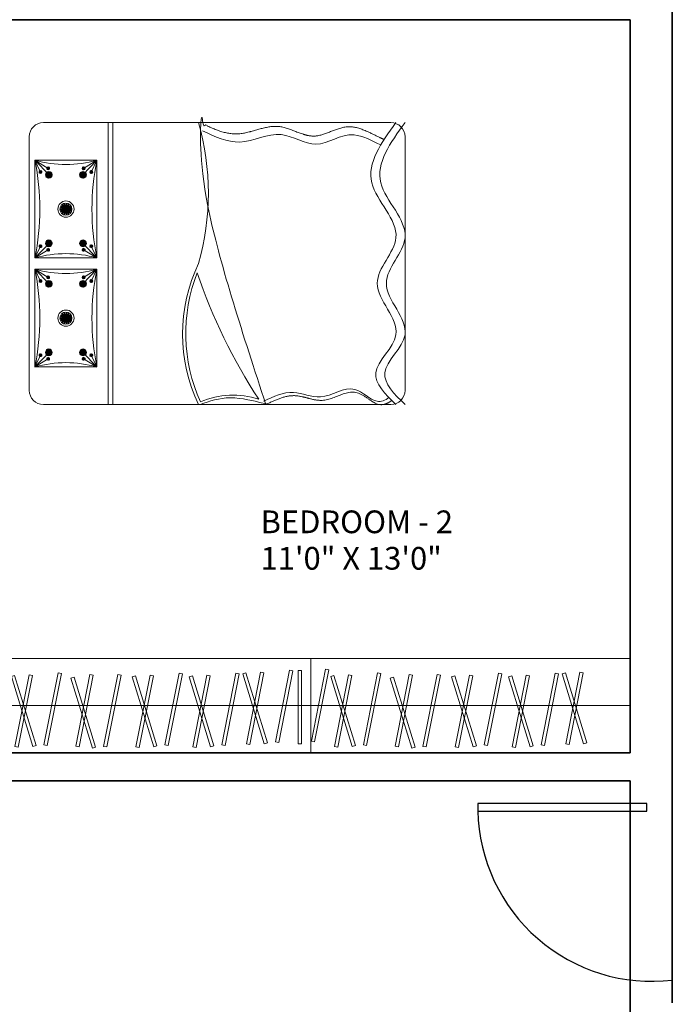
# Model space of a CAD drawing. Units: inches. Extents: x -61 to 1599, y -1316 to 257.
# Tile 203 of 204: x 1384 to 1523, y -61 to 149. Entities that reach past the tile are written whole.
import ezdxf

# ---------------------------------------------------------------- set-up
doc = ezdxf.new("R2010")
doc.units = ezdxf.units.IN
doc.header["$MEASUREMENT"] = 0
for name, color, linetype, lineweight in [('A-AREA-IDEN', 1, 'Continuous', 18), ('A-FLOR-CASE', 8, 'Continuous', 18), ('DOORS', 2, 'Continuous', 25), ('FURNITURE', 83, 'Continuous', 18), ('WALLS', 4, 'Continuous', 35)]:
    doc.layers.add(name, color=color, linetype=linetype, lineweight=lineweight)
doc.layers.add('LT', color=8, linetype='Continuous')
doc.styles.get("Standard").update_dxf_attribs({"font": 'arial.ttf'})

# ---------------------------------------------------------------- blocks, each defined once
blk = doc.blocks.new('DOOR-SWING-36-ALT')
blk.add_lwpolyline([(0, 0), (-36, 0), (-36, -1.58), (0, -1.58)], close=True)
blk.add_arc((1.08, -0.74), 37.09, 181.2913, 276.6905)
blk = doc.blocks.new('WARDROBE-HANGING')
blk.add_line((10.05, 0), (10.05, 68))
for points in [[(20.09, 0), (0, 0), (0, 68), (20.09, 68)], [(2.48, 67.85), (17.75, 64.85), (17.61, 64.14), (2.34, 67.15)], [(1.32, 62.96), (16.59, 59.95), (16.45, 59.25), (1.19, 62.25)], [(1.35, 59.16), (16.22, 63.73), (16.43, 63.04), (1.56, 58.47)], [(1.71, 56.78), (16.98, 53.78), (16.84, 53.07), (1.57, 56.08)], [(1, 46.47), (15.87, 51.04), (16.08, 50.35), (1.21, 45.78)], [(1.39, 50.01), (16.66, 47.01), (16.52, 46.3), (1.26, 49.31)], [(1.36, 44.09), (16.63, 41.09), (16.49, 40.38), (1.23, 43.38)], [(1.28, 33.41), (16.16, 37.98), (16.37, 37.29), (1.49, 32.72)], [(1.26, 37.2), (16.53, 34.2), (16.39, 33.49), (1.12, 36.5)], [(1.65, 31.03), (16.92, 28.03), (16.78, 27.32), (1.51, 30.32)], [(1.28, 21.3), (16.15, 25.87), (16.36, 25.18), (1.49, 20.61)], [(1.26, 25.09), (16.53, 22.09), (16.39, 21.38), (1.12, 24.39)], [(1.65, 18.92), (16.91, 15.92), (16.78, 15.21), (1.51, 18.21)], [(1.91, 13.69), (17.17, 10.68), (17.04, 9.98), (1.77, 12.98)], [(1.93, 9.89), (16.8, 14.46), (17.01, 13.77), (2.14, 9.2)], [(2.29, 7.51), (17.56, 4.51), (17.42, 3.8), (2.16, 6.81)], [(17.49, 1.96), (1.93, 1.96), (1.93, 2.68), (17.49, 2.68)]]:
    blk.add_lwpolyline(points, close=True)
blk = doc.blocks.new('WARDROBE-HANGING-4')
blk.add_line((68, 10.05), (0, 10.05))
for points in [[(68, 20.09), (68, 0), (0, 0), (0, 20.09)], [(0.15, 2.48), (3.15, 17.75), (3.86, 17.61), (0.85, 2.34)], [(11.22, 1.71), (14.22, 16.98), (14.93, 16.84), (11.92, 1.57)], [(36.97, 1.65), (39.97, 16.92), (40.68, 16.78), (37.68, 1.51)], [(49.08, 1.65), (52.08, 16.91), (52.79, 16.78), (49.79, 1.51)], [(58.11, 1.93), (53.54, 16.8), (54.23, 17.01), (58.8, 2.14)], [(54.31, 1.91), (57.32, 17.17), (58.02, 17.04), (55.02, 1.77)], [(8.84, 1.35), (4.27, 16.22), (4.96, 16.43), (9.53, 1.56)], [(5.04, 1.32), (8.05, 16.59), (8.75, 16.45), (5.75, 1.19)], [(21.53, 1), (16.96, 15.87), (17.65, 16.08), (22.22, 1.21)], [(17.99, 1.39), (20.99, 16.66), (21.7, 16.52), (18.69, 1.25)], [(23.91, 1.36), (26.91, 16.63), (27.62, 16.49), (24.62, 1.23)], [(34.59, 1.28), (30.02, 16.16), (30.71, 16.37), (35.28, 1.49)], [(30.8, 1.26), (33.8, 16.53), (34.51, 16.39), (31.5, 1.12)], [(46.7, 1.28), (42.13, 16.15), (42.82, 16.36), (47.39, 1.49)], [(42.91, 1.26), (45.91, 16.53), (46.62, 16.39), (43.61, 1.12)]]:
    blk.add_lwpolyline(points, close=True)
blk = doc.blocks.new('*U100')
at = {"layer": 'LT'}
blk.add_line((0, 0.15), (0, -0.15), dxfattribs=at)
for centre, start, end in [((0.44, 0), 160.9983, 199.0017), ((-0.44, 0), 340.9983, 19.0017)]:
    blk.add_arc(centre, 0.468, start, end, dxfattribs=at)
blk = doc.blocks.new('*U101')
at = {"layer": 'LT', "transparency": 16777216}
for p, rotation in [((-57.96, -16.37), 96), ((-57.96, -16.31), 72), ((-57.94, -16.43), 120), ((-57.93, -16.26), 48.00000000000001), ((-57.9, -16.48), 144), ((-57.87, -16.22), 24), ((-57.84, -16.51), 168.0000000000001), ((-57.75, -16.22), 336), ((-57.78, -16.51), 192), ((-57.7, -16.26), 312), ((-57.72, -16.48), 216), ((-57.68, -16.43), 240), ((-57.67, -16.31), 288), ((-57.66, -16.37), 264)]:
    blk.add_blockref('*U100', p, dxfattribs=dict(at, rotation=rotation))
blk.add_blockref('*U100', (-57.81, -16.21), dxfattribs=at)
blk = doc.blocks.new('*U104')
at = {"layer": 'LT'}
blk.add_line((0, 0.15), (0, -0.15), dxfattribs=at)
for centre, start, end in [((0.44, 0), 160.9983, 199.0017), ((-0.44, 0), 340.9983, 19.0017)]:
    blk.add_arc(centre, 0.468, start, end, dxfattribs=at)
blk = doc.blocks.new('*U105')
at = {"layer": 'LT', "transparency": 16777216}
for p, rotation in [((-57.96, -16.37), 96), ((-57.96, -16.31), 72), ((-57.94, -16.43), 120), ((-57.93, -16.26), 48.00000000000001), ((-57.9, -16.48), 144), ((-57.87, -16.22), 24), ((-57.84, -16.51), 168.0000000000001), ((-57.75, -16.22), 336), ((-57.78, -16.51), 192), ((-57.7, -16.26), 312), ((-57.72, -16.48), 216), ((-57.68, -16.43), 240), ((-57.67, -16.31), 288), ((-57.66, -16.37), 264)]:
    blk.add_blockref('*U104', p, dxfattribs=dict(at, rotation=rotation))
blk.add_blockref('*U104', (-57.81, -16.21), dxfattribs=at)
blk = doc.blocks.new('*U71')
at = {"layer": 'LT'}
blk.add_line((0, 0.15), (0, -0.15), dxfattribs=at)
for centre, start, end in [((0.44, 0), 160.9983, 199.0017), ((-0.44, 0), 340.9983, 19.0017)]:
    blk.add_arc(centre, 0.468, start, end, dxfattribs=at)
blk = doc.blocks.new('*U58')
at = {"layer": 'LT', "transparency": 16777216}
for p, rotation in [((-57.96, -16.37), 96), ((-57.96, -16.31), 72), ((-57.94, -16.43), 120), ((-57.93, -16.26), 48.00000000000001), ((-57.9, -16.48), 144), ((-57.87, -16.22), 24), ((-57.84, -16.51), 168.0000000000001), ((-57.75, -16.22), 336), ((-57.78, -16.51), 192), ((-57.7, -16.26), 312), ((-57.72, -16.48), 216), ((-57.68, -16.43), 240), ((-57.67, -16.31), 288), ((-57.66, -16.37), 264)]:
    blk.add_blockref('*U71', p, dxfattribs=dict(at, rotation=rotation))
blk.add_blockref('*U71', (-57.81, -16.21), dxfattribs=at)
blk = doc.blocks.new('*U61')
at = {"layer": 'LT'}
blk.add_line((0, 0.15), (0, -0.15), dxfattribs=at)
for centre, start, end in [((0.44, 0), 160.9983, 199.0017), ((-0.44, 0), 340.9983, 19.0017)]:
    blk.add_arc(centre, 0.468, start, end, dxfattribs=at)
blk = doc.blocks.new('*U62')
at = {"layer": 'LT', "transparency": 16777216}
for p, rotation in [((-57.96, -16.37), 96), ((-57.96, -16.31), 72), ((-57.94, -16.43), 120), ((-57.93, -16.26), 48.00000000000001), ((-57.9, -16.48), 144), ((-57.87, -16.22), 24), ((-57.84, -16.51), 168.0000000000001), ((-57.75, -16.22), 336), ((-57.78, -16.51), 192), ((-57.7, -16.26), 312), ((-57.72, -16.48), 216), ((-57.68, -16.43), 240), ((-57.67, -16.31), 288), ((-57.66, -16.37), 264)]:
    blk.add_blockref('*U61', p, dxfattribs=dict(at, rotation=rotation))
blk.add_blockref('*U61', (-57.81, -16.21), dxfattribs=at)
blk = doc.blocks.new('*U94')
at = {"layer": 'LT'}
blk.add_line((0, 0.36), (0, -0.36), dxfattribs=at)
for centre, start, end in [((1.04, 0), 160.9983, 199.0017), ((-1.04, 0), 340.9983, 19.0017)]:
    blk.add_arc(centre, 1.1, start, end, dxfattribs=at)
blk = doc.blocks.new('*U95')
at = {"layer": 'LT', "transparency": 16777216}
for p, rotation in [((-136.32, -38.51), 96), ((-136.3, -38.36), 72), ((-136.27, -38.65), 120), ((-136.23, -38.23), 48.00000000000001), ((-136.17, -38.76), 144), ((-136.11, -38.14), 23.99999999999999), ((-136.04, -38.82), 168.0000000000001), ((-135.82, -38.14), 336.0000000000001), ((-135.89, -38.82), 191.9999999999999), ((-135.75, -38.76), 216), ((-135.69, -38.23), 312), ((-135.65, -38.65), 240), ((-135.62, -38.36), 288.0000000000001), ((-135.6, -38.51), 264)]:
    blk.add_blockref('*U94', p, dxfattribs=dict(at, rotation=rotation))
blk.add_blockref('*U94', (-135.96, -38.11), dxfattribs=at)
blk = doc.blocks.new('*U57')
at = {"layer": 'LT'}
blk.add_line((0, 0.36), (0, -0.36), dxfattribs=at)
for centre, start, end in [((1.04, 0), 160.9983, 199.0017), ((-1.04, 0), 340.9983, 19.0017)]:
    blk.add_arc(centre, 1.1, start, end, dxfattribs=at)
blk = doc.blocks.new('*U99')
at = {"layer": 'LT', "transparency": 16777216}
for p, rotation in [((-136.32, -38.51), 96), ((-136.3, -38.36), 72), ((-136.27, -38.65), 120), ((-136.23, -38.23), 48.00000000000001), ((-136.17, -38.76), 144), ((-136.11, -38.14), 23.99999999999999), ((-136.04, -38.82), 168.0000000000001), ((-135.82, -38.14), 336.0000000000001), ((-135.89, -38.82), 191.9999999999999), ((-135.75, -38.76), 216), ((-135.69, -38.23), 312), ((-135.65, -38.65), 240), ((-135.62, -38.36), 288.0000000000001), ((-135.6, -38.51), 264)]:
    blk.add_blockref('*U57', p, dxfattribs=dict(at, rotation=rotation))
blk.add_blockref('*U57', (-135.96, -38.11), dxfattribs=at)
blk = doc.blocks.new('*U80')
at = {"layer": 'LT'}
blk.add_line((0, 0.36), (0, -0.36), dxfattribs=at)
for centre, start, end in [((1.04, 0), 160.9983, 199.0017), ((-1.04, 0), 340.9983, 19.0017)]:
    blk.add_arc(centre, 1.1, start, end, dxfattribs=at)
blk = doc.blocks.new('*U96')
at = {"layer": 'LT', "transparency": 16777216}
for p, rotation in [((-136.32, -38.51), 96), ((-136.3, -38.36), 72), ((-136.27, -38.65), 120), ((-136.23, -38.23), 48.00000000000001), ((-136.17, -38.76), 144), ((-136.11, -38.14), 23.99999999999999), ((-136.04, -38.82), 168.0000000000001), ((-135.82, -38.14), 336.0000000000001), ((-135.89, -38.82), 191.9999999999999), ((-135.75, -38.76), 216), ((-135.69, -38.23), 312), ((-135.65, -38.65), 240), ((-135.62, -38.36), 288.0000000000001), ((-135.6, -38.51), 264)]:
    blk.add_blockref('*U80', p, dxfattribs=dict(at, rotation=rotation))
blk.add_blockref('*U80', (-135.96, -38.11), dxfattribs=at)
blk = doc.blocks.new('*U69')
at = {"layer": 'LT'}
blk.add_line((0, 0.36), (0, -0.36), dxfattribs=at)
for centre, start, end in [((1.04, 0), 160.9983, 199.0017), ((-1.04, 0), 340.9983, 19.0017)]:
    blk.add_arc(centre, 1.1, start, end, dxfattribs=at)
blk = doc.blocks.new('*U70')
at = {"layer": 'LT', "transparency": 16777216}
for p, rotation in [((-136.32, -38.51), 96), ((-136.3, -38.36), 72), ((-136.27, -38.65), 120), ((-136.23, -38.23), 48.00000000000001), ((-136.17, -38.76), 144), ((-136.11, -38.14), 23.99999999999999), ((-136.04, -38.82), 168.0000000000001), ((-135.82, -38.14), 336.0000000000001), ((-135.89, -38.82), 191.9999999999999), ((-135.75, -38.76), 216), ((-135.69, -38.23), 312), ((-135.65, -38.65), 240), ((-135.62, -38.36), 288.0000000000001), ((-135.6, -38.51), 264)]:
    blk.add_blockref('*U69', p, dxfattribs=dict(at, rotation=rotation))
blk.add_blockref('*U69', (-135.96, -38.11), dxfattribs=at)
blk = doc.blocks.new('*U102')
at = {"layer": 'LT'}
blk.add_line((0, 0.15), (0, -0.15), dxfattribs=at)
for centre, start, end in [((0.44, 0), 160.9983, 199.0017), ((-0.44, 0), 340.9983, 19.0017)]:
    blk.add_arc(centre, 0.468, start, end, dxfattribs=at)
blk = doc.blocks.new('*U103')
at = {"layer": 'LT', "transparency": 16777216}
for p, rotation in [((-57.96, -16.37), 96), ((-57.96, -16.31), 72), ((-57.94, -16.43), 120), ((-57.93, -16.26), 48.00000000000001), ((-57.9, -16.48), 144), ((-57.87, -16.22), 24), ((-57.84, -16.51), 168.0000000000001), ((-57.75, -16.22), 336), ((-57.78, -16.51), 192), ((-57.7, -16.26), 312), ((-57.72, -16.48), 216), ((-57.68, -16.43), 240), ((-57.67, -16.31), 288), ((-57.66, -16.37), 264)]:
    blk.add_blockref('*U102', p, dxfattribs=dict(at, rotation=rotation))
blk.add_blockref('*U102', (-57.81, -16.21), dxfattribs=at)
blk = doc.blocks.new('*U55')
at = {"layer": 'LT'}
blk.add_line((0, 0.15), (0, -0.15), dxfattribs=at)
for centre, start, end in [((0.44, 0), 160.9983, 199.0017), ((-0.44, 0), 340.9983, 19.0017)]:
    blk.add_arc(centre, 0.468, start, end, dxfattribs=at)
blk = doc.blocks.new('*U56')
at = {"layer": 'LT', "transparency": 16777216}
for p, rotation in [((-57.96, -16.37), 96), ((-57.96, -16.31), 72), ((-57.94, -16.43), 120), ((-57.93, -16.26), 48.00000000000001), ((-57.9, -16.48), 144), ((-57.87, -16.22), 24), ((-57.84, -16.51), 168.0000000000001), ((-57.75, -16.22), 336), ((-57.78, -16.51), 192), ((-57.7, -16.26), 312), ((-57.72, -16.48), 216), ((-57.68, -16.43), 240), ((-57.67, -16.31), 288), ((-57.66, -16.37), 264)]:
    blk.add_blockref('*U55', p, dxfattribs=dict(at, rotation=rotation))
blk.add_blockref('*U55', (-57.81, -16.21), dxfattribs=at)
blk = doc.blocks.new('*U59')
at = {"layer": 'LT'}
blk.add_line((0, 0.15), (0, -0.15), dxfattribs=at)
for centre, start, end in [((0.44, 0), 160.9983, 199.0017), ((-0.44, 0), 340.9983, 19.0017)]:
    blk.add_arc(centre, 0.468, start, end, dxfattribs=at)
blk = doc.blocks.new('*U60')
at = {"layer": 'LT', "transparency": 16777216}
for p, rotation in [((-57.96, -16.37), 96), ((-57.96, -16.31), 72), ((-57.94, -16.43), 120), ((-57.93, -16.26), 48.00000000000001), ((-57.9, -16.48), 144), ((-57.87, -16.22), 24), ((-57.84, -16.51), 168.0000000000001), ((-57.75, -16.22), 336), ((-57.78, -16.51), 192), ((-57.7, -16.26), 312), ((-57.72, -16.48), 216), ((-57.68, -16.43), 240), ((-57.67, -16.31), 288), ((-57.66, -16.37), 264)]:
    blk.add_blockref('*U59', p, dxfattribs=dict(at, rotation=rotation))
blk.add_blockref('*U59', (-57.81, -16.21), dxfattribs=at)
blk = doc.blocks.new('*U67')
at = {"layer": 'LT'}
blk.add_line((0, 0.15), (0, -0.15), dxfattribs=at)
for centre, start, end in [((0.44, 0), 160.9983, 199.0017), ((-0.44, 0), 340.9983, 19.0017)]:
    blk.add_arc(centre, 0.468, start, end, dxfattribs=at)
blk = doc.blocks.new('*U68')
at = {"layer": 'LT', "transparency": 16777216}
for p, rotation in [((-57.96, -16.37), 96), ((-57.96, -16.31), 72), ((-57.94, -16.43), 120), ((-57.93, -16.26), 48.00000000000001), ((-57.9, -16.48), 144), ((-57.87, -16.22), 24), ((-57.84, -16.51), 168.0000000000001), ((-57.75, -16.22), 336), ((-57.78, -16.51), 192), ((-57.7, -16.26), 312), ((-57.72, -16.48), 216), ((-57.68, -16.43), 240), ((-57.67, -16.31), 288), ((-57.66, -16.37), 264)]:
    blk.add_blockref('*U67', p, dxfattribs=dict(at, rotation=rotation))
blk.add_blockref('*U67', (-57.81, -16.21), dxfattribs=at)
blk = doc.blocks.new('*U106')
at = {"layer": 'LT'}
blk.add_line((0, 0.64), (0, -0.64), dxfattribs=at)
for centre, start, end in [((1.87, 0), 160.9983, 199.0017), ((-1.87, 0), 340.9983, 19.0017)]:
    blk.add_arc(centre, 1.97, start, end, dxfattribs=at)
blk = doc.blocks.new('*U93')
at = {"layer": 'LT', "transparency": 16777216}
for p, rotation in [((-244.36, -69.03), 96), ((-244.33, -68.76), 72), ((-244.28, -69.28), 120), ((-244.2, -68.53), 48.00000000000001), ((-244.1, -69.48), 144), ((-243.98, -68.38), 23.99999999999999), ((-243.86, -69.59), 168), ((-243.59, -69.59), 192), ((-243.46, -68.38), 336.0000000000001), ((-243.34, -69.48), 216), ((-243.25, -68.53), 312), ((-243.17, -69.28), 240), ((-243.11, -68.76), 288), ((-243.08, -69.03), 264)]:
    blk.add_blockref('*U106', p, dxfattribs=dict(at, rotation=rotation))
blk.add_blockref('*U106', (-243.72, -68.32), dxfattribs=at)
blk = doc.blocks.new('*U63')
at = {"layer": 'LT'}
blk.add_line((0, 0.64), (0, -0.64), dxfattribs=at)
for centre, start, end in [((1.87, 0), 160.9983, 199.0017), ((-1.87, 0), 340.9983, 19.0017)]:
    blk.add_arc(centre, 1.97, start, end, dxfattribs=at)
blk = doc.blocks.new('*U64')
at = {"layer": 'LT', "transparency": 16777216}
for p, rotation in [((-244.36, -69.03), 96), ((-244.33, -68.76), 72), ((-244.28, -69.28), 120), ((-244.2, -68.53), 48.00000000000001), ((-244.1, -69.48), 144), ((-243.98, -68.38), 23.99999999999999), ((-243.86, -69.59), 168), ((-243.59, -69.59), 192), ((-243.46, -68.38), 336.0000000000001), ((-243.34, -69.48), 216), ((-243.25, -68.53), 312), ((-243.17, -69.28), 240), ((-243.11, -68.76), 288), ((-243.08, -69.03), 264)]:
    blk.add_blockref('*U63', p, dxfattribs=dict(at, rotation=rotation))
blk.add_blockref('*U63', (-243.72, -68.32), dxfattribs=at)
blk = doc.blocks.new('*U83')
at = {"layer": 'LT'}
blk.add_line((0, 0.36), (0, -0.36), dxfattribs=at)
for centre, start, end in [((1.04, 0), 160.9983, 199.0017), ((-1.04, 0), 340.9983, 19.0017)]:
    blk.add_arc(centre, 1.1, start, end, dxfattribs=at)
blk = doc.blocks.new('*U84')
at = {"layer": 'LT', "transparency": 16777216}
for p, rotation in [((-136.32, -38.51), 96), ((-136.3, -38.36), 72), ((-136.27, -38.65), 120), ((-136.23, -38.23), 48.00000000000001), ((-136.17, -38.76), 144), ((-136.11, -38.14), 23.99999999999999), ((-136.04, -38.82), 168.0000000000001), ((-135.82, -38.14), 336.0000000000001), ((-135.89, -38.82), 191.9999999999999), ((-135.75, -38.76), 216), ((-135.69, -38.23), 312), ((-135.65, -38.65), 240), ((-135.62, -38.36), 288.0000000000001), ((-135.6, -38.51), 264)]:
    blk.add_blockref('*U83', p, dxfattribs=dict(at, rotation=rotation))
blk.add_blockref('*U83', (-135.96, -38.11), dxfattribs=at)
blk = doc.blocks.new('*U74')
at = {"layer": 'LT'}
blk.add_line((0, 0.36), (0, -0.36), dxfattribs=at)
for centre, start, end in [((1.04, 0), 160.9983, 199.0017), ((-1.04, 0), 340.9983, 19.0017)]:
    blk.add_arc(centre, 1.1, start, end, dxfattribs=at)
blk = doc.blocks.new('*U75')
at = {"layer": 'LT', "transparency": 16777216}
for p, rotation in [((-136.32, -38.51), 96), ((-136.3, -38.36), 72), ((-136.27, -38.65), 120), ((-136.23, -38.23), 48.00000000000001), ((-136.17, -38.76), 144), ((-136.11, -38.14), 23.99999999999999), ((-136.04, -38.82), 168.0000000000001), ((-135.82, -38.14), 336.0000000000001), ((-135.89, -38.82), 191.9999999999999), ((-135.75, -38.76), 216), ((-135.69, -38.23), 312), ((-135.65, -38.65), 240), ((-135.62, -38.36), 288.0000000000001), ((-135.6, -38.51), 264)]:
    blk.add_blockref('*U74', p, dxfattribs=dict(at, rotation=rotation))
blk.add_blockref('*U74', (-135.96, -38.11), dxfattribs=at)
blk = doc.blocks.new('*U65')
at = {"layer": 'LT'}
blk.add_line((0, 0.36), (0, -0.36), dxfattribs=at)
for centre, start, end in [((1.04, 0), 160.9983, 199.0017), ((-1.04, 0), 340.9983, 19.0017)]:
    blk.add_arc(centre, 1.1, start, end, dxfattribs=at)
blk = doc.blocks.new('*U66')
at = {"layer": 'LT', "transparency": 16777216}
for p, rotation in [((-136.32, -38.51), 96), ((-136.3, -38.36), 72), ((-136.27, -38.65), 120), ((-136.23, -38.23), 48.00000000000001), ((-136.17, -38.76), 144), ((-136.11, -38.14), 23.99999999999999), ((-136.04, -38.82), 168.0000000000001), ((-135.82, -38.14), 336.0000000000001), ((-135.89, -38.82), 191.9999999999999), ((-135.75, -38.76), 216), ((-135.69, -38.23), 312), ((-135.65, -38.65), 240), ((-135.62, -38.36), 288.0000000000001), ((-135.6, -38.51), 264)]:
    blk.add_blockref('*U65', p, dxfattribs=dict(at, rotation=rotation))
blk.add_blockref('*U65', (-135.96, -38.11), dxfattribs=at)
blk = doc.blocks.new('*U85')
at = {"layer": 'LT'}
blk.add_line((0, 0.36), (0, -0.36), dxfattribs=at)
for centre, start, end in [((1.04, 0), 160.9983, 199.0017), ((-1.04, 0), 340.9983, 19.0017)]:
    blk.add_arc(centre, 1.1, start, end, dxfattribs=at)
blk = doc.blocks.new('*U86')
at = {"layer": 'LT', "transparency": 16777216}
for p, rotation in [((-136.32, -38.51), 96), ((-136.3, -38.36), 72), ((-136.27, -38.65), 120), ((-136.23, -38.23), 48.00000000000001), ((-136.17, -38.76), 144), ((-136.11, -38.14), 23.99999999999999), ((-136.04, -38.82), 168.0000000000001), ((-135.82, -38.14), 336.0000000000001), ((-135.89, -38.82), 191.9999999999999), ((-135.75, -38.76), 216), ((-135.69, -38.23), 312), ((-135.65, -38.65), 240), ((-135.62, -38.36), 288.0000000000001), ((-135.6, -38.51), 264)]:
    blk.add_blockref('*U85', p, dxfattribs=dict(at, rotation=rotation))
blk.add_blockref('*U85', (-135.96, -38.11), dxfattribs=at)
blk = doc.blocks.new('*U78')
at = {"layer": 'LT'}
blk.add_line((0, 0.15), (0, -0.15), dxfattribs=at)
for centre, start, end in [((0.44, 0), 160.9983, 199.0017), ((-0.44, 0), 340.9983, 19.0017)]:
    blk.add_arc(centre, 0.468, start, end, dxfattribs=at)
blk = doc.blocks.new('*U79')
at = {"layer": 'LT', "transparency": 16777216}
for p, rotation in [((-57.96, -16.37), 96), ((-57.96, -16.31), 72), ((-57.94, -16.43), 120), ((-57.93, -16.26), 48.00000000000001), ((-57.9, -16.48), 144), ((-57.87, -16.22), 24), ((-57.84, -16.51), 168.0000000000001), ((-57.75, -16.22), 336), ((-57.78, -16.51), 192), ((-57.7, -16.26), 312), ((-57.72, -16.48), 216), ((-57.68, -16.43), 240), ((-57.67, -16.31), 288), ((-57.66, -16.37), 264)]:
    blk.add_blockref('*U78', p, dxfattribs=dict(at, rotation=rotation))
blk.add_blockref('*U78', (-57.81, -16.21), dxfattribs=at)
blk = doc.blocks.new('*U72')
at = {"layer": 'LT'}
blk.add_line((0, 0.15), (0, -0.15), dxfattribs=at)
for centre, start, end in [((0.44, 0), 160.9983, 199.0017), ((-0.44, 0), 340.9983, 19.0017)]:
    blk.add_arc(centre, 0.468, start, end, dxfattribs=at)
blk = doc.blocks.new('*U73')
at = {"layer": 'LT', "transparency": 16777216}
for p, rotation in [((-57.96, -16.37), 96), ((-57.96, -16.31), 72), ((-57.94, -16.43), 120), ((-57.93, -16.26), 48.00000000000001), ((-57.9, -16.48), 144), ((-57.87, -16.22), 24), ((-57.84, -16.51), 168.0000000000001), ((-57.75, -16.22), 336), ((-57.78, -16.51), 192), ((-57.7, -16.26), 312), ((-57.72, -16.48), 216), ((-57.68, -16.43), 240), ((-57.67, -16.31), 288), ((-57.66, -16.37), 264)]:
    blk.add_blockref('*U72', p, dxfattribs=dict(at, rotation=rotation))
blk.add_blockref('*U72', (-57.81, -16.21), dxfattribs=at)
blk = doc.blocks.new('*U89')
at = {"layer": 'LT'}
blk.add_line((0, 0.15), (0, -0.15), dxfattribs=at)
for centre, start, end in [((0.44, 0), 160.9983, 199.0017), ((-0.44, 0), 340.9983, 19.0017)]:
    blk.add_arc(centre, 0.468, start, end, dxfattribs=at)
blk = doc.blocks.new('*U90')
at = {"layer": 'LT', "transparency": 16777216}
for p, rotation in [((-57.96, -16.37), 96), ((-57.96, -16.31), 72), ((-57.94, -16.43), 120), ((-57.93, -16.26), 48.00000000000001), ((-57.9, -16.48), 144), ((-57.87, -16.22), 24), ((-57.84, -16.51), 168.0000000000001), ((-57.75, -16.22), 336), ((-57.78, -16.51), 192), ((-57.7, -16.26), 312), ((-57.72, -16.48), 216), ((-57.68, -16.43), 240), ((-57.67, -16.31), 288), ((-57.66, -16.37), 264)]:
    blk.add_blockref('*U89', p, dxfattribs=dict(at, rotation=rotation))
blk.add_blockref('*U89', (-57.81, -16.21), dxfattribs=at)
blk = doc.blocks.new('*U97')
at = {"layer": 'LT'}
blk.add_line((0, 0.15), (0, -0.15), dxfattribs=at)
for centre, start, end in [((0.44, 0), 160.9983, 199.0017), ((-0.44, 0), 340.9983, 19.0017)]:
    blk.add_arc(centre, 0.468, start, end, dxfattribs=at)
blk = doc.blocks.new('*U98')
at = {"layer": 'LT', "transparency": 16777216}
for p, rotation in [((-57.96, -16.37), 96), ((-57.96, -16.31), 72), ((-57.94, -16.43), 120), ((-57.93, -16.26), 48.00000000000001), ((-57.9, -16.48), 144), ((-57.87, -16.22), 24), ((-57.84, -16.51), 168.0000000000001), ((-57.75, -16.22), 336), ((-57.78, -16.51), 192), ((-57.7, -16.26), 312), ((-57.72, -16.48), 216), ((-57.68, -16.43), 240), ((-57.67, -16.31), 288), ((-57.66, -16.37), 264)]:
    blk.add_blockref('*U97', p, dxfattribs=dict(at, rotation=rotation))
blk.add_blockref('*U97', (-57.81, -16.21), dxfattribs=at)
blk = doc.blocks.new('*U76')
at = {"layer": 'LT'}
blk.add_line((0, 0.15), (0, -0.15), dxfattribs=at)
for centre, start, end in [((0.44, 0), 160.9983, 199.0017), ((-0.44, 0), 340.9983, 19.0017)]:
    blk.add_arc(centre, 0.468, start, end, dxfattribs=at)
blk = doc.blocks.new('*U77')
at = {"layer": 'LT', "transparency": 16777216}
for p, rotation in [((-57.96, -16.37), 96), ((-57.96, -16.31), 72), ((-57.94, -16.43), 120), ((-57.93, -16.26), 48.00000000000001), ((-57.9, -16.48), 144), ((-57.87, -16.22), 24), ((-57.84, -16.51), 168.0000000000001), ((-57.75, -16.22), 336), ((-57.78, -16.51), 192), ((-57.7, -16.26), 312), ((-57.72, -16.48), 216), ((-57.68, -16.43), 240), ((-57.67, -16.31), 288), ((-57.66, -16.37), 264)]:
    blk.add_blockref('*U76', p, dxfattribs=dict(at, rotation=rotation))
blk.add_blockref('*U76', (-57.81, -16.21), dxfattribs=at)
blk = doc.blocks.new('*U81')
at = {"layer": 'LT'}
blk.add_line((0, 0.15), (0, -0.15), dxfattribs=at)
for centre, start, end in [((0.44, 0), 160.9983, 199.0017), ((-0.44, 0), 340.9983, 19.0017)]:
    blk.add_arc(centre, 0.468, start, end, dxfattribs=at)
blk = doc.blocks.new('*U82')
at = {"layer": 'LT', "transparency": 16777216}
for p, rotation in [((-57.96, -16.37), 96), ((-57.96, -16.31), 72), ((-57.94, -16.43), 120), ((-57.93, -16.26), 48.00000000000001), ((-57.9, -16.48), 144), ((-57.87, -16.22), 24), ((-57.84, -16.51), 168.0000000000001), ((-57.75, -16.22), 336), ((-57.78, -16.51), 192), ((-57.7, -16.26), 312), ((-57.72, -16.48), 216), ((-57.68, -16.43), 240), ((-57.67, -16.31), 288), ((-57.66, -16.37), 264)]:
    blk.add_blockref('*U81', p, dxfattribs=dict(at, rotation=rotation))
blk.add_blockref('*U81', (-57.81, -16.21), dxfattribs=at)
blk = doc.blocks.new('*U87')
at = {"layer": 'LT'}
blk.add_line((0, 0.15), (0, -0.15), dxfattribs=at)
for centre, start, end in [((0.44, 0), 160.9983, 199.0017), ((-0.44, 0), 340.9983, 19.0017)]:
    blk.add_arc(centre, 0.468, start, end, dxfattribs=at)
blk = doc.blocks.new('*U88')
at = {"layer": 'LT', "transparency": 16777216}
for p, rotation in [((-57.96, -16.37), 96), ((-57.96, -16.31), 72), ((-57.94, -16.43), 120), ((-57.93, -16.26), 48.00000000000001), ((-57.9, -16.48), 144), ((-57.87, -16.22), 24), ((-57.84, -16.51), 168.0000000000001), ((-57.75, -16.22), 336), ((-57.78, -16.51), 192), ((-57.7, -16.26), 312), ((-57.72, -16.48), 216), ((-57.68, -16.43), 240), ((-57.67, -16.31), 288), ((-57.66, -16.37), 264)]:
    blk.add_blockref('*U87', p, dxfattribs=dict(at, rotation=rotation))
blk.add_blockref('*U87', (-57.81, -16.21), dxfattribs=at)
blk = doc.blocks.new('*U91')
at = {"layer": 'LT'}
blk.add_line((0, 0.15), (0, -0.15), dxfattribs=at)
for centre, start, end in [((0.44, 0), 160.9983, 199.0017), ((-0.44, 0), 340.9983, 19.0017)]:
    blk.add_arc(centre, 0.468, start, end, dxfattribs=at)
blk = doc.blocks.new('*U92')
at = {"layer": 'LT', "transparency": 16777216}
for p, rotation in [((-57.96, -16.37), 96), ((-57.96, -16.31), 72), ((-57.94, -16.43), 120), ((-57.93, -16.26), 48.00000000000001), ((-57.9, -16.48), 144), ((-57.87, -16.22), 24), ((-57.84, -16.51), 168.0000000000001), ((-57.75, -16.22), 336), ((-57.78, -16.51), 192), ((-57.7, -16.26), 312), ((-57.72, -16.48), 216), ((-57.68, -16.43), 240), ((-57.67, -16.31), 288), ((-57.66, -16.37), 264)]:
    blk.add_blockref('*U91', p, dxfattribs=dict(at, rotation=rotation))
blk.add_blockref('*U91', (-57.81, -16.21), dxfattribs=at)
blk = doc.blocks.new('BED-DOUBLE-COMPACT')
for p, q in [((16.8, 60.04), (16.8, 0.04)), ((17.8, 60.04), (17.8, 0.04)), ((1.2, 52.04), (14.4, 52.04)), ((1.2, 52.04), (2.4, 49.53)), ((1.2, 52.04), (4.2, 48.93)), ((1.2, 52.04), (4.03, 50.31)), ((4.03, 50.31), (4.33, 50.31)), ((11.57, 50.31), (11.27, 50.31)), ((14.4, 52.04), (11.4, 48.93)), ((14.4, 52.04), (11.57, 50.31)), ((14.4, 52.04), (13.2, 49.53)), ((14.4, 31.24), (14.4, 52.04)), ((2.4, 49.53), (2.7, 49.53)), ((4.16, 48.92), (4.88, 48.92)), ((11.44, 48.92), (10.72, 48.92)), ((13.2, 49.53), (12.9, 49.53)), ((7.8, 41.64), (9.09, 41.64)), ((1.2, 31.24), (4.2, 34.34)), ((1.2, 31.24), (2.4, 33.74)), ((2.4, 33.74), (2.7, 33.74)), ((4.16, 34.35), (4.88, 34.35)), ((11.44, 34.35), (10.72, 34.35)), ((14.4, 31.24), (11.4, 34.34)), ((13.2, 33.74), (12.9, 33.74)), ((14.4, 31.24), (13.2, 33.74)), ((1.2, 31.24), (4.03, 32.96)), ((4.03, 32.96), (4.33, 32.96)), ((11.57, 32.96), (11.27, 32.96)), ((14.4, 31.24), (11.57, 32.96)), ((1.2, 31.24), (1.2, 31.24)), ((1.2, 28.84), (14.4, 28.84)), ((1.2, 28.84), (2.4, 26.33)), ((1.2, 28.84), (4.2, 25.73)), ((1.2, 28.84), (4.03, 27.11)), ((14.4, 28.84), (11.4, 25.73)), ((14.4, 28.84), (11.57, 27.11)), ((14.4, 28.84), (13.2, 26.33)), ((14.4, 8.04), (14.4, 28.84)), ((2.4, 26.33), (2.7, 26.33)), ((4.03, 27.11), (4.33, 27.11)), ((4.16, 25.72), (4.88, 25.72)), ((11.44, 25.72), (10.72, 25.72)), ((11.57, 27.11), (11.27, 27.11)), ((13.2, 26.33), (12.9, 26.33)), ((7.8, 18.44), (9.09, 18.44)), ((1.2, 8.04), (4.2, 11.14)), ((1.2, 8.04), (2.4, 10.54)), ((2.4, 10.54), (2.7, 10.54)), ((4.16, 11.15), (4.88, 11.15)), ((11.44, 11.15), (10.72, 11.15)), ((14.4, 8.04), (11.4, 11.14)), ((13.2, 10.54), (12.9, 10.54)), ((14.4, 8.04), (13.2, 10.54)), ((1.2, 8.04), (4.03, 9.76)), ((4.03, 9.76), (4.33, 9.76)), ((11.57, 9.76), (11.27, 9.76)), ((14.4, 8.04), (11.57, 9.76)), ((1.2, 8.04), (1.2, 8.04))]:
    blk.add_line(p, q)
for points in [[(77, 60.04), (3, 60.04, 0.414214), (0, 57.04), (0, 3.04, 0.414214), (3, 0.04), (77, 0.04, 0.414214), (80, 3.04), (80, 57.04, 0.414214)], [(4.33, 50.31, 0.167358), (4.03, 50.31, 0.167358)], [(11.57, 50.31, 0.167358), (11.27, 50.31, 0.167358)], [(2.7, 49.53, 0.167358), (2.4, 49.53, 0.167358)], [(4.88, 48.92, 0.167358), (4.16, 48.92, 0.167358)], [(11.44, 48.92, 0.167358), (10.72, 48.92, 0.167358)], [(13.2, 49.53, 0.167358), (12.9, 49.53, 0.167358)], [(7.8, 41.64, 0.167358), (9.09, 41.64, 0.167358)], [(2.4, 33.74, 0.167358), (2.7, 33.74, 0.167358)], [(4.16, 34.35, 0.167358), (4.88, 34.35, 0.167358)], [(10.72, 34.35, 0.167358), (11.44, 34.35, 0.167358)], [(4.03, 32.96, 0.167358), (4.33, 32.96, 0.167358)], [(11.27, 32.96, 0.167358), (11.57, 32.96, 0.167358)], [(35.77, 28.09, 0.064396), (48.86, 1.19, 0.181766), (36.45, 0.6, -0.202767)], [(2.7, 26.33, 0.167358), (2.4, 26.33, 0.167358)], [(4.33, 27.11, 0.167358), (4.03, 27.11, 0.167358)], [(4.88, 25.72, 0.167358), (4.16, 25.72, 0.167358)], [(11.44, 25.72, 0.167358), (10.72, 25.72, 0.167358)], [(11.57, 27.11, 0.167358), (11.27, 27.11, 0.167358)], [(13.2, 26.33, 0.167358), (12.9, 26.33, 0.167358)], [(7.8, 18.44, 0.167358), (9.09, 18.44, 0.167358)], [(2.4, 10.54, 0.167358), (2.7, 10.54, 0.167358)], [(4.16, 11.15, 0.167358), (4.88, 11.15, 0.167358)], [(10.72, 11.15, 0.167358), (11.44, 11.15, 0.167358)], [(4.03, 9.76, 0.167358), (4.33, 9.76, 0.167358)], [(11.27, 9.76, 0.167358), (11.57, 9.76, 0.167358)]]:
    blk.add_lwpolyline(points, format="xyb", close=True)
blk.add_lwpolyline([(36, 0.04, -0.22309), (36, 30.04, 0.142156), (36, 60.04)], format="xyb")
for points in [[(14.4, 31.24), (1.2, 31.24), (1.2, 52.04), (14.4, 52.04), (14.4, 31.24), (1.2, 31.24), (1.2, 52.04)], [(14.4, 8.04), (1.2, 8.04), (1.2, 28.84)]]:
    blk.add_lwpolyline(points)
for centre, radius in [((4.03, 50.31), 0.305), ((11.57, 50.31), 0.305), ((2.4, 49.53), 0.305), ((4.16, 48.92), 0.717), ((11.44, 48.92), 0.717), ((13.2, 49.53), 0.305), ((7.8, 41.64), 1.72), ((7.8, 41.64), 1.29), ((2.4, 33.74), 0.305), ((4.16, 34.35), 0.717), ((11.44, 34.35), 0.717), ((13.2, 33.74), 0.305), ((4.03, 32.96), 0.305), ((11.57, 32.96), 0.305), ((4.03, 27.11), 0.305), ((11.57, 27.11), 0.305), ((2.4, 26.33), 0.305), ((4.16, 25.72), 0.717), ((11.44, 25.72), 0.717), ((13.2, 26.33), 0.305), ((7.8, 18.44), 1.72), ((7.8, 18.44), 1.29), ((2.4, 10.54), 0.305), ((4.16, 11.15), 0.717), ((11.44, 11.15), 0.717), ((13.2, 10.54), 0.305), ((4.03, 9.76), 0.305), ((11.57, 9.76), 0.305)]:
    blk.add_circle(centre, radius)
for centre, radius, start, end in [((-49.23, 41.64), 51.49, 348.3468, 11.6532), ((7.8, 75.06), 23.95, 254.0046, 285.9954), ((64.83, 41.64), 51.49, 168.3468, 191.6532), ((13.05, 33.3), 0.468, 70.9983, 109.0017), ((13.05, 34.18), 0.468, 250.9983, 289.0017), ((7.8, 8.21), 23.95, 74.0046, 105.9954), ((-49.23, 18.44), 51.49, 348.3468, 11.6532), ((7.8, 51.86), 23.95, 254.0046, 285.9954), ((64.83, 18.44), 51.49, 168.3468, 191.6532), ((13.05, 10.1), 0.468, 70.9983, 109.0017), ((13.05, 10.98), 0.468, 250.9983, 289.0017), ((7.8, -14.99), 23.95, 74.0046, 105.9954)]:
    blk.add_arc(centre, radius, start, end)
for points, weights, knots in [([(50.36, 0.04), (44.31, 9.08), (39.57, 18.88), (36.25, 29.24), (36.33, 29.43), (36.41, 29.62), (36.5, 29.81), (39.38, 39.75), (39.36, 50.11), (36.43, 60.04), (39.05, 58.77), (44.5, 56.15), (52.79, 61.02), (60.85, 55.2), (67.65, 61.05), (73.39, 57.36), (75.56, 56.45)], [1, 0.993520320424, 0.993520320424, 1, 0.99997444972, 0.99997444972, 1, 0.973174868659, 0.973174868659, 1, 1, 1, 1, 1, 1, 1, 1], [0, 0, 0, 0, 0.279074, 0.279074, 0.279074, 0.296584, 0.296584, 0.296584, 0.865868, 0.865868, 0.865868, 9.142578, 18.107734, 25.769226, 34.110801, 40.441511, 40.441511, 40.441511, 40.441511]), ([(36.38, 0.04), (40.9, 1.99), (45.83, 1.99), (50.36, 0.04), (52.47, 1.05), (56.42, 2.94), (63, -0.48), (69.27, 4.67), (73.92, -0.77), (76.3, 0.25), (77.18, 0.91)], [1, 0.945466318698, 0.945466318698, 1, 1, 1, 1, 1, 1, 1, 1], [0, 0, 0, 0, 0.814571, 0.814571, 0.814571, 7.464247, 13.266353, 20.788537, 26.138745, 29.321895, 29.321895, 29.321895, 29.321895])]:
    blk.add_rational_spline(points, weights, degree=3, knots=knots)
for points, knots in [([(78.07, 0.04), (75.8, 2.26), (70.92, 7.04), (82.19, 15.5), (70.03, 25.56), (82.2, 36.26), (68.97, 47.49), (74.96, 55.75), (78.07, 60.04)], [0, 0, 0, 0, 7.980285, 17.179806, 28.830278, 39.318084, 52.078264, 65.891546, 65.891546, 65.891546, 65.891546]), ([(80, 0.04), (77.73, 2.26), (72.85, 7.04), (84.12, 15.5), (71.96, 25.56), (84.13, 36.26), (70.9, 47.49), (76.89, 55.75), (80, 60.04)], [0, 0, 0, 0, 7.980285, 17.179806, 28.830278, 39.318084, 52.078264, 65.891546, 65.891546, 65.891546, 65.891546]), ([(36.91, 58.31), (39.53, 57.05), (44.98, 54.43), (53.27, 59.3), (61.33, 53.48), (67.78, 59.03), (72.97, 56.17), (74.83, 55.28)], [0, 0, 0, 0, 8.27671, 17.241866, 24.903358, 33.244933, 38.427294, 38.427294, 38.427294, 38.427294]), ([(49.89, 0.74), (52, 1.75), (55.95, 3.65), (62.54, 0.23), (68.8, 5.38), (73.4, -0.01), (75.74, 0.92), (76.58, 1.52)], [0, 0, 0, 0, 6.649676, 12.451782, 19.973966, 25.324174, 28.349676, 28.349676, 28.349676, 28.349676])]:
    blk.add_open_spline(points, degree=3, knots=knots)
blk.add_open_spline([(80, 56.78), (80.02, 56.81), (80.03, 56.83), (80.05, 56.85)], degree=3)
at = {"xscale": -1}
for name, p, rotation in [('*U68', (-12.33, -7.5), 90), ('*U62', (-13.96, -8.28), 90), ('*U70', (-34.31, -87.04), 90), ('*U66', (49.91, 170.31), 270), ('*U88', (29.56, 91.55), 270), ('*U90', (27.93, 90.77), 270), ('*U56', (-12.33, -30.7), 90), ('*U105', (-13.96, -31.48), 90), ('*U99', (-34.31, -110.24), 90), ('*U84', (49.91, 147.11), 270), ('*U77', (29.56, 68.35), 270), ('*U79', (27.93, 67.57), 270)]:
    blk.add_blockref(name, p, dxfattribs=dict(at, rotation=rotation))
for name, p, rotation in [('*U98', (27.93, -7.5), 270), ('*U86', (49.91, -87.04), 270), ('*U92', (29.56, -8.28), 270), ('*U64', (-61.16, 285.36), 89.99999999999999), ('*U58', (-13.96, 91.55), 89.99999999999999), ('*U96', (-34.31, 170.31), 89.99999999999999), ('*U60', (-12.33, 90.77), 89.99999999999999), ('*U73', (27.93, -30.7), 270), ('*U75', (49.91, -110.24), 270), ('*U82', (29.56, -31.48), 270), ('*U93', (-61.16, 262.16), 89.99999999999999), ('*U101', (-13.96, 68.35), 89.99999999999999), ('*U95', (-34.31, 147.11), 89.99999999999999), ('*U103', (-12.33, 67.57), 89.99999999999999)]:
    blk.add_blockref(name, p, dxfattribs=dict(rotation=rotation))

msp = doc.modelspace()

# ---------------------------------------------------------------- linework, layer by layer
at = {"layer": 'WALLS'}
for p, q in [((1522.7028, 157.6771), (1522.7028, 34.831)), ((1381.7028, 148.6771), (1513.7028, 148.6771)), ((1513.7028, 148.6771), (1513.7028, -7.3229)), ((1522.7028, -60.5493), (1522.7028, 34.831)), ((1375.7028, -7.3229), (1513.7028, -7.3229)), ((1375.7028, -13.3229), (1513.7028, -13.3229)), ((1513.7028, -13.3229), (1513.7028, -175.3229))]:
    msp.add_line(p, q, dxfattribs=at)

# ---------------------------------------------------------------- block references
at = {"layer": 'A-FLOR-CASE', "rotation": 90.00000000000033}
msp.add_blockref('WARDROBE-HANGING', (1445.7029, -7.3231), dxfattribs=at)
at = {"layer": 'A-FLOR-CASE'}
msp.add_blockref('WARDROBE-HANGING-4', (1445.703, -7.323), dxfattribs=at)
at = {"layer": 'DOORS'}
msp.add_blockref('DOOR-SWING-36-ALT', (1517.3028, -18.1418), dxfattribs=at)
at = {"layer": 'FURNITURE'}
msp.add_blockref('BED-DOUBLE-COMPACT', (1385.794, 66.733), dxfattribs=at)

# ---------------------------------------------------------------- texts
at = {"layer": 'A-AREA-IDEN'}
for s, p in [('BEDROOM - 2', (1435.0332, 39.4006)), ('11\'0" X 13\'0"', (1435.0332, 31.6383))]:
    msp.add_text(s, height=4.832098, dxfattribs=at).set_placement(p)

doc.saveas('drawing.dxf')
